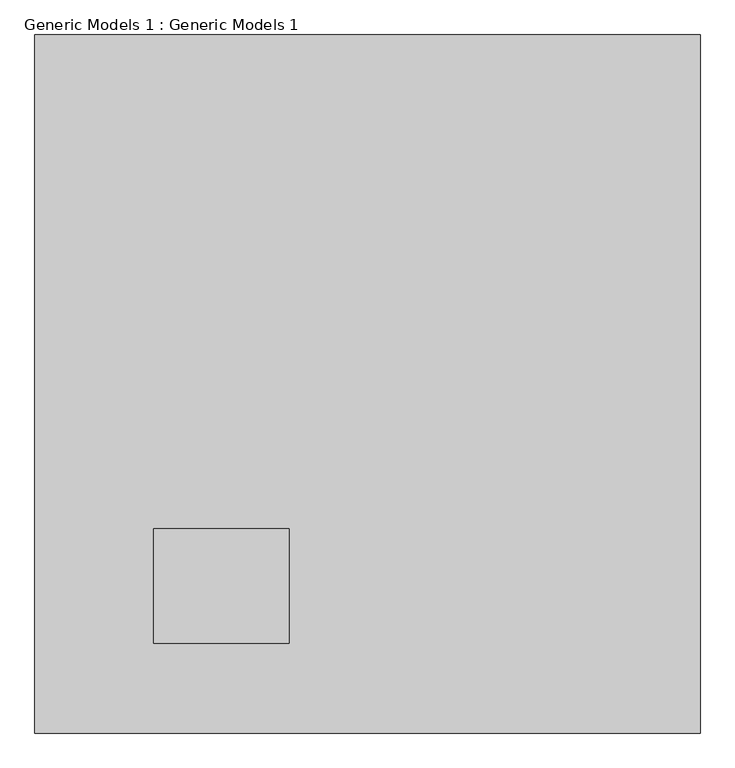
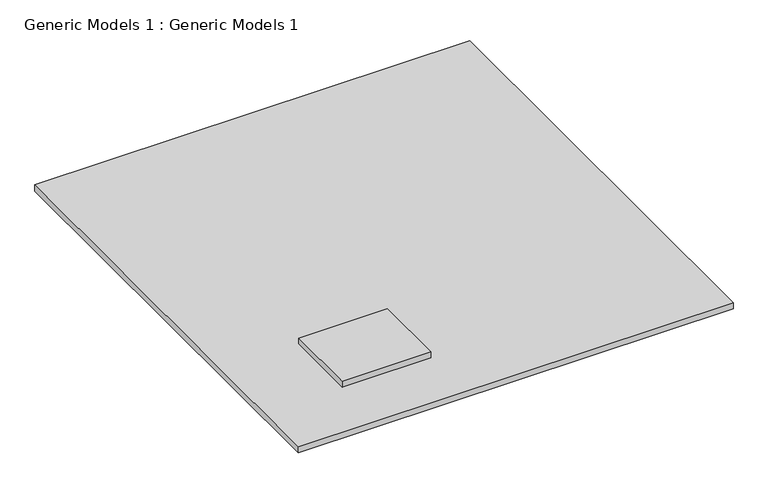
"""IFC4 building model written with IfcOpenShell, lengths in millimetres: proxy geometry, Generic Models 1 : Generic Models 1."""

from ifc_helpers import new_model, si_unit, frame, origin, origin_with_axes, place, context, project, spatial, polyline, outline, extrude, source, transform, mapped, element, save


def generic_models_1_generic_models_1_93a2076a(model_context):
    return source(origin(), model_context, "Body", "SweptSolid", [
        extrude(outline(polyline([(-1655.9127168, 3965.6627723), (-1655.9127168, -17641.446149), (-22255.3579891, -17641.446149), (-22255.3579891, 3965.6627723), (-1655.9127168, 3965.6627723)])), frame((0.0, 0.0, -304.8), z_axis=(0.0, 0.0, 1.0), x_axis=(1.0, 0.0, 0.0)), (0.0, 0.0, 1.0), 304.8),
        extrude(outline(polyline([(-14380.8761094, -11316.846149), (-14380.8761094, -14860.146149), (-18571.8761094, -14860.146149), (-18571.8761094, -11316.846149), (-14380.8761094, -11316.846149)])), origin_with_axes(), (0.0, 0.0, 1.0), 304.8),
    ])


if __name__ == "__main__":
    model = new_model("IFC4")
    model_context = context("Model", 3, world=origin())
    ifc_project = project(units=[si_unit("LENGTHUNIT", "METRE", prefix="MILLI")], contexts=[model_context])
    site = spatial("IfcSite", under=ifc_project)
    building = spatial("IfcBuilding", under=site)
    placement = place(None, origin())
    generic_models_1_generic_models_1_shape = generic_models_1_generic_models_1_93a2076a(model_context)
    element("IfcBuildingElementProxy", 1, Name="Generic Models 1 : Generic Models 1", ObjectType="Generic Models 1 : Generic Models 1", at=placement, inside=building, context=model_context, shape_type="MappedRepresentation", body=[
        mapped(generic_models_1_generic_models_1_shape, transform((0.0, 0.0, 0.0), x_axis=(1.0, 0.0, 0.0), y_axis=(0.0, 1.0, 0.0), z_axis=(0.0, 0.0, 1.0))),
    ])
    save(model, "model.ifc")
